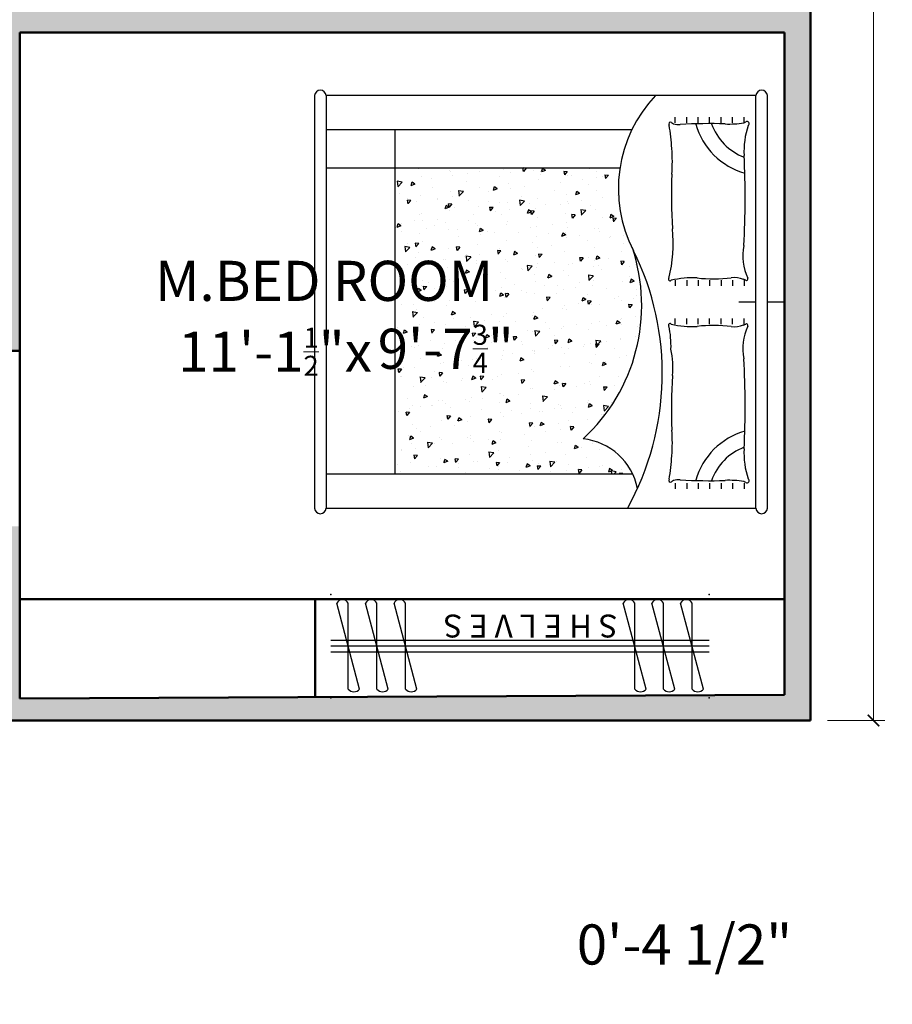
# Model space of a CAD drawing. Units: inches. Extents: x 4508 to 5907, y 877 to 1592.
# Tile 8 of 20: x 5392 to 5544, y 877 to 1049. Entities that reach past the tile are written whole.
import ezdxf

# ---------------------------------------------------------------- set-up
doc = ezdxf.new("R2010")
doc.units = ezdxf.units.IN
doc.layers.get('DEFPOINTS').update_dxf_attribs({"color": 8})
for name, color, linetype, lineweight in [('A-ANNO-DIMS', 2, 'Continuous', 18), ('A-FURN', 24, 'Continuous', 18), ('A-WALL', 7, 'Continuous', 50), ('A-WALL-PATT', 8, 'Continuous', 13)]:
    doc.layers.add(name, color=color, linetype=linetype, lineweight=lineweight)
doc.layers.add('furniture', color=24, linetype='Continuous')
doc.styles.get("Standard").update_dxf_attribs({"font": 'arial.ttf'})
doc.dimstyles.new('details', dxfattribs={"dimtxt": 5, "dimasz": 2, "dimexe": 2, "dimexo": 3, "dimgap": 1, "dimtad": 0, "dimdec": 1, "dimzin": 0, "dimdsep": 46, "dimlunit": 4, "dimtxsty": 'Standard', "dimblk": 'ARCHTICK', "dimcen": 3, "dimclrd": 256, "dimclre": 256, "dimclrt": 256, "dimadec": 0, "dimazin": 0, "dimtfac": 0.5, "dimtdec": 1, "dimtofl": 0, "dimtmove": 0, "dimatfit": 3, "dimldrblk": 'CLOSEDBLANK', "dimfxl": 2, "dimtolj": 1, "dimtzin": 0, "dimlwd": -1, "dimlwe": -1, "dimarcsym": 0})
doc.dimstyles.new('text', dxfattribs={"dimtxt": 7, "dimasz": 0, "dimexe": 3, "dimexo": 3, "dimgap": 0, "dimtad": 1, "dimtih": 1, "dimtoh": 1, "dimzin": 3, "dimdsep": 46, "dimlunit": 4, "dimtxsty": 'Standard', "dimblk": 'CLOSEDBLANK', "dimcen": 3, "dimse1": 1, "dimse2": 1, "dimsd1": 1, "dimsd2": 1, "dimclrd": 256, "dimclre": 256, "dimclrt": 256, "dimadec": 0, "dimazin": 0, "dimtfac": 0.5, "dimtofl": 0, "dimtmove": 0, "dimatfit": 3, "dimfxl": 3, "dimtolj": 1, "dimtzin": 0, "dimlwd": -1, "dimlwe": -1, "dimarcsym": 0})

# ---------------------------------------------------------------- blocks, each defined once
blk = doc.blocks.new('bed')
at = {"layer": 'furniture'}
h = blk.add_hatch(dxfattribs=at)
h.set_pattern_fill('AR-CONC', color=256, angle=-90, style=0)
h.set_pattern_definition([(320, (0, 2.38), (-0.6275, -7.1726), [0.75, -8.25]), (265, (0, 2.38), (7.5219, 1.3875), [0.6, -6.6]), (10.451, (-0.052, 1.782), (6.8944, -5.7851), [0.6374, -7.0114]), (316.184, (2, 2.38), (-1.6552, -10.6724), [1.125, -12.375]), (6.636, (1.862, 1.491), (9.7412, -9.3466), [0.9561, -10.5171]), (261.184, (2, 2.38), (9.7412, -9.3466), [0.9, -9.9]), (291, (1.5, 1.38), (-4.0262, -5.96907), [0.75, -8.25]), (236, (1.5, 1.38), (7.2515, -2.43315), [0.6, -6.6]), (341.451, (1.1645, 0.8826), (3.2253, -8.4022), [0.6374, -7.0114]), (307.5, (0, 2.38), (3.32894, -0.1216), [0, -6.52, 0, -6.7, 0, -6.625]), (277.5, (0, 2.38), (3.94412, -2.6307), [0, -3.82, 0, -6.37, 0, -2.525]), (237.5, (0, 4.61), (-0.22555, -5.33822), [0, -2.5, 0, -7.8, 0, -10.35]), (227.5, (0, 5.61), (1.00105, -5.83186), [0, -3.25, 0, -5.18, 0, -7.35])])
h.paths.add_polyline_path([(30.01, -68), (30.01, -26.5, 0.263043), (23.9, -35.15, 0.293424), (-9.18, -26.47, -0.156683), (-23.39, -28.72), (-23.39, -68)])
for p, q in [((0, -3), (0, 0)), ((36.01, -3), (-36.01, -3)), ((-36.01, -5), (-36.01, -80)), ((36.01, -5), (-36.01, -5)), ((0, -8), (0, -5)), ((36.01, -80), (36.01, -5)), ((-31.24, -7.07), (-32.24, -7.07)), ((-3.81, -7.07), (-2.81, -7.07)), ((3.89, -7.07), (2.89, -7.07)), ((31.63, -7.07), (32.63, -7.07)), ((-31.24, -9.07), (-32.24, -9.07)), ((-3.81, -9.07), (-2.81, -9.07)), ((3.89, -9.07), (2.89, -9.07)), ((31.63, -9.07), (32.63, -9.07)), ((-31.24, -11.07), (-32.24, -11.07)), ((-3.81, -11.07), (-2.81, -11.07)), ((3.89, -11.07), (2.89, -11.07)), ((31.63, -11.07), (32.63, -11.07)), ((-31.24, -13.07), (-32.24, -13.07)), ((-3.81, -13.07), (-2.81, -13.07)), ((3.89, -13.07), (2.89, -13.07)), ((31.63, -13.07), (32.63, -13.07)), ((-31.24, -15.07), (-32.24, -15.07)), ((-3.81, -15.07), (-2.81, -15.07)), ((3.89, -15.07), (2.89, -15.07)), ((31.63, -15.07), (32.63, -15.07)), ((-31.24, -17.07), (-32.24, -17.07)), ((-3.81, -17.07), (-2.81, -17.07)), ((3.89, -17.07), (2.89, -17.07)), ((31.63, -17.07), (32.63, -17.07)), ((-31.24, -19.07), (-32.24, -19.07)), ((-3.81, -19.07), (-2.81, -19.07)), ((3.89, -19.07), (2.89, -19.07)), ((31.63, -19.07), (32.63, -19.07)), ((-36.01, -80), (36.01, -80)), ((-36.01, -82), (36.01, -82))]:
    blk.add_line(p, q, dxfattribs=at)
at = {"layer": 'furniture', "ltscale": 5}
blk.add_line((-30.01, -26.66), (-30.01, -80), dxfattribs=at)
at = {"layer": 'furniture', "ltscale": 7}
blk.add_line((30.01, -80), (30.01, -26.5), dxfattribs=at)
at = {"layer": 'furniture', "ltscale": 0.3}
for p, q in [((-23.39, -80), (-23.39, -28.72)), ((-30.01, -68), (30.01, -68))]:
    blk.add_line(p, q, dxfattribs=at)
at = {"layer": 'furniture'}
for centre, radius, start, end in [((-35.95, -4), 1, 93.3831, 266.6169), ((35.95, -4), 1, 273.3831, 86.6169), ((-31.1, -6.57), 0.382, 35.8976, 208.6272), ((-44.44, -13.85), 14.82, 27.1629, 28.6272), ((-26.35, 6.68), 13.76, 251.1782, 273.3982), ((-8.03, 2.03), 9.29, 258.896, 294.7184), ((-4.03, -6.67), 0.282, 335.7259, 114.303), ((3.22, -9.94), 7.68, 155.7259, 159.0146), ((4.11, -6.67), 0.282, 65.697, 204.2741), ((-3.14, -9.94), 7.68, 20.9854, 24.2741), ((8.12, 2.03), 9.29, 245.2816, 281.104), ((26.43, 6.68), 13.76, 266.6018, 288.8218), ((31.18, -6.57), 0.382, 331.3728, 144.1024), ((44.53, -13.85), 14.82, 151.3728, 152.8371), ((-46.76, -9.65), 15.72, 357.4804, 9.3956), ((-34.45, -3.51), 9.85, 289.8695, 338.9843), ((-34.45, -3.51), 12.47, 286.0319, 344.1205), ((-18.02, -163.6), 156.72, 87.0032, 92.7497), ((0.25, -8.8), 4.49, 159.0146, 186.273), ((-0.17, -8.8), 4.49, 353.727, 20.9854), ((18.1, -163.6), 156.72, 87.2503, 92.9968), ((34.54, -3.51), 12.47, 195.8795, 253.9681), ((34.54, -3.51), 9.85, 201.0157, 250.1305), ((46.84, -9.65), 15.72, 170.6044, 182.5196), ((-32.82, -12.44), 28.78, 354.3784, 6.273), ((32.9, -12.44), 28.78, 173.727, 185.6216), ((-28.62, 31.03), 42.31, 266.4836, 266.6487), ((54.88, -13.16), 85.99, 178.1209, 183.3613), ((-54.8, -13.16), 85.99, 356.6387, 1.8791), ((28.7, 31.03), 42.31, 273.3513, 273.5164), ((12.28, -16.11), 16.48, 177.0317, 192.8678), ((-12.19, -16.11), 16.48, 347.1322, 2.9683), ((-34.13, -18.41), 3.18, 342.7809, 3.755), ((34.21, -18.41), 3.18, 176.245, 197.2191), ((-31.05, -19.91), 0.291, 147.6219, 311.9343), ((-33.2, -18.55), 2.25, 327.6219, 339.2246), ((-24.4, -58.01), 38.42, 93.5164, 99.6766), ((-24.52, -56.06), 36.48, 86.4836, 93.5164), ((-18.49, 70.49), 90.23, 267.5921, 273.6329), ((-10.31, -44.95), 25.52, 75.952, 95.5452), ((-3.95, -19.99), 0.265, 231.9005, 52.8902), ((4.03, -19.99), 0.265, 127.1098, 308.0995), ((7.57, -34.68), 14.87, 87.3976, 103.1191), ((11.44, -34.81), 15.32, 84.694, 102.0355), ((18.57, 70.49), 90.23, 266.3671, 272.4079), ((24.6, -56.06), 36.48, 86.4836, 93.5164), ((24.48, -58.01), 38.42, 80.3234, 86.4836), ((31.13, -19.91), 0.291, 228.0657, 32.3781), ((33.28, -18.55), 2.25, 200.7754, 212.3781), ((12.51, -69.71), 48.38, 60.9345, 116.3227), ((-19.79, -5.47), 23.53, 226.4061, 297.4441), ((0.6, -56.57), 31.65, 42.5874, 108.5034), ((34.61, -36.23), 10.76, 101.1719, 174.259), ((-35.95, -81), 1, 93.3831, 266.6169), ((35.95, -81), 1, 273.3831, 86.6169)]:
    blk.add_arc(centre, radius, start, end, dxfattribs=at)
blk = doc.blocks.new('*D109')
at = {"layer": 'DEFPOINTS', "color": 0, "transparency": 16777216}
for p in [(5460.86, 1046.7), (5455.62, 930.84), (5466.29, 930.84)]:
    blk.add_point(p, dxfattribs=at)
at = {"layer": 'A-ANNO-DIMS', "color": 0, "transparency": 16777216, "insert": (5466.29, 991.53), "char_height": 7, "width": 32.6217, "attachment_point": 5}
blk.add_mtext('\\A1;9\'-7{\\H0.5x;\\S3/4;}"', dxfattribs=at)
blk = doc.blocks.new('_ClosedBlank')
at = {"color": 0, "lineweight": -2}
for p, q in [((-1, 0.167), (0, 0)), ((-1, 0.167), (-1, -0.167)), ((0, 0), (-1, -0.167))]:
    blk.add_line(p, q, dxfattribs=at)
blk = doc.blocks.new('*D110')
at = {"layer": 'DEFPOINTS', "color": 0, "transparency": 16777216}
for p in [(5525.4, 986.86), (5391.95, 982.69), (5525.4, 975.67)]:
    blk.add_point(p, dxfattribs=at)
at = {"layer": 'A-ANNO-DIMS', "color": 0, "transparency": 16777216, "insert": (5436.51, 996.85), "char_height": 7, "attachment_point": 5}
blk.add_mtext('\\A1;        M.BED ROOM\\P11\'-1{\\H0.5x;\\S1/2;}"x', dxfattribs=at)
blk = doc.blocks.new('hangers')
at = {"layer": 'furniture'}
for p, q in [((1, 7.5), (5, -7.5)), ((3, 7.5), (3, -7.5)), ((6, 7.5), (10, -7.5)), ((8, 7.5), (8, -7.5)), ((11, 7.5), (15, -7.5)), ((13, 7.5), (13, -7.5)), ((51, 7.5), (55, -7.5)), ((53, 7.5), (53, -7.5)), ((56, 7.5), (60, -7.5)), ((58, 7.5), (58, -7.5)), ((61, 7.5), (65, -7.5)), ((63, 7.5), (63, -7.5)), ((66, 1), (0, 1)), ((0, 0), (66, 0)), ((0, -1), (66, -1))]:
    blk.add_line(p, q, dxfattribs=at)
for centre, radius, start, end in [((2, 6.62), 1.33, 41.2884, 138.7116), ((7, 6.62), 1.33, 41.2884, 138.7116), ((12, 6.62), 1.33, 41.2884, 138.7116), ((52, 6.62), 1.33, 41.2884, 138.7116), ((57, 6.62), 1.33, 41.2884, 138.7116), ((62, 6.62), 1.33, 41.2884, 138.7116), ((4, -7.08), 1.08, 202.5549, 337.4451), ((9, -7.08), 1.08, 202.5549, 337.4451), ((14, -7.08), 1.08, 202.5549, 337.4451), ((54, -7.08), 1.08, 202.5549, 337.4451), ((59, -7.08), 1.08, 202.5549, 337.4451), ((64, -7.08), 1.08, 202.5549, 337.4451)]:
    blk.add_arc(centre, radius, start, end, dxfattribs=at)
for p in [(0, 9), (66, 9), (0, -9), (66, -9)]:
    blk.add_point(p, dxfattribs=at)
blk.add_text('S H E L V E S', height=4, dxfattribs=at).set_placement((16, -5.52))
blk = doc.blocks.new('_ArchTick')
at = {"color": 0, "linetype": 'ByBlock', "const_width": 0.15}
blk.add_lwpolyline([(-0.5, -0.5), (0.5, 0.5)], dxfattribs=at)
blk = doc.blocks.new('*D113')
at = {"layer": 'A-ANNO-DIMS', "color": 0, "transparency": 16777216}
for p, q in [((5532.9, 1574.7), (5542.92, 1574.7)), ((5540.92, 1574.7), (5540.92, 1255.95)), ((5540.92, 926.7), (5540.92, 1245.46)), ((5532.9, 926.7), (5542.92, 926.7))]:
    blk.add_line(p, q, dxfattribs=at)
at = {"layer": 'DEFPOINTS', "color": 0, "transparency": 16777216}
for p in [(5529.9, 1574.7), (5540.92, 1574.7), (5529.9, 926.7)]:
    blk.add_point(p, dxfattribs=at)
at = {"layer": 'A-ANNO-DIMS', "color": 0, "transparency": 16777216, "xscale": 2, "yscale": 2, "zscale": 2}
for p, rotation in [((5540.92, 1574.7), 90), ((5540.92, 926.7), 270)]:
    blk.add_blockref('_ArchTick', p, dxfattribs=dict(at, rotation=rotation))
at = {"layer": 'A-ANNO-DIMS', "color": 0, "transparency": 16777216, "insert": (5540.92, 1250.7), "char_height": 5, "attachment_point": 5, "rotation": 90}
blk.add_mtext("\\A1;54'", dxfattribs=at)
blk = doc.blocks.new('*D189')
at = {"layer": 'DEFPOINTS', "color": 0, "transparency": 16777216}
for p in [(5525.4, 931.18), (5529.9, 926.7), (5529.9, 883.98)]:
    blk.add_point(p, dxfattribs=at)
at = {"layer": 'A-ANNO-DIMS', "transparency": 16777216, "insert": (5507.94, 887.6), "char_height": 7, "attachment_point": 5}
blk.add_mtext('\\A1;0\'-4 1/2"', dxfattribs=at)

msp = doc.modelspace()

# ---------------------------------------------------------------- hatches: boundary and pattern name
at = {"layer": 'A-WALL-PATT'}
h = msp.add_hatch(color=256, dxfattribs=at)
h.dxf.hatch_style = 1
h.paths.add_polyline_path([(5529.903, 1303.204), (5388.02, 1303.204), (5388.02, 1294.204), (5391.903, 1294.204), (5391.903, 1205.704), (5396.403, 1205.704), (5396.403, 1294.204), (5489.403, 1294.204), (5489.403, 1256.139), (5493.903, 1256.139), (5493.903, 1294.204), (5529.903, 1294.204)], flags=17)
h.paths.add_polyline_path([(5346.02, 1303.204), (5322.903, 1303.204), (5322.903, 1321.388), (5313.903, 1321.388), (5313.903, 1303.204), (5259.903, 1303.204), (5259.903, 1381.204), (5313.903, 1381.204), (5313.903, 1359.674), (5322.903, 1359.674), (5322.903, 1381.204), (5338.979, 1381.204), (5338.979, 1390.204), (5331.903, 1390.204), (5331.903, 1442.704), (5255.403, 1442.704), (5255.403, 1570.204), (5387.403, 1570.204), (5387.403, 1541.271), (5391.903, 1541.271), (5391.903, 1570.204), (5483.403, 1570.204), (5483.403, 1498.204), (5391.903, 1498.204), (5391.903, 1509.559), (5387.403, 1509.559), (5387.403, 1390.204), (5380.979, 1390.204), (5380.979, 1381.204), (5387.403, 1381.204), (5529.903, 1381.204), (5529.903, 1498.204), (5487.903, 1498.204), (5487.903, 1570.204), (5529.903, 1570.204), (5529.903, 1574.704), (5250.903, 1574.704), (5250.903, 991.204), (5310.903, 991.204), (5310.903, 926.704), (5529.903, 926.704), (5529.903, 1210.204), (5525.403, 1210.204), (5525.403, 1103.704), (5499.903, 1103.704), (5499.903, 1210.204), (5493.903, 1210.204), (5493.903, 1256.139), (5489.403, 1256.139), (5489.403, 1210.204), (5461.584, 1210.204), (5461.584, 1205.704), (5495.403, 1205.704), (5495.403, 1103.704), (5436.903, 1103.704), (5436.903, 1051.204), (5391.954, 1051.204), (5391.954, 1103.03), (5391.954, 1107.53), (5255.403, 1108.204), (5255.403, 1294.204), (5346.02, 1294.204)])
h.paths.add_polyline_path([(5255.403, 1390.204), (5255.403, 1398.204), (5255.403, 1438.204), (5257.903, 1438.204), (5258.903, 1438.204), (5327.403, 1438.204), (5327.403, 1390.204), (5325.903, 1390.204)], flags=16)
h.paths.add_polyline_path([(5288.757, 1390.704), (5288.757, 1390.204), (5292.173, 1390.204), (5292.173, 1390.704)], flags=0)
h.paths.add_polyline_path([(5289.965, 1391.606), (5289.965, 1396.645), (5289.903, 1396.645), (5289.903, 1397.319), (5288.849, 1398.862), (5288.849, 1398.8), (5288.983, 1398.748), (5288.983, 1399.204), (5289.091, 1399.204), (5292.081, 1399.204), (5292.081, 1398.665), (5291.946, 1398.665), (5291.027, 1397.319), (5291.027, 1396.645), (5290.965, 1396.645), (5290.965, 1391.606)], flags=0)
h.paths.add_polyline_path([(5288.849, 1399.069, 2.6374395), (5289.056, 1398.835), (5289.117, 1399.087, 0.9346155)], flags=0)
h.paths.add_polyline_path([(5290.061, 1398.665), (5290.061, 1399.204), (5290.038, 1398.975)], flags=0)
h.paths.add_polyline_path([(5291.946, 1398.934, -1), (5291.946, 1398.665)], flags=0)
h.paths.add_polyline_path([(5289.414, 1398.967), (5289.414, 1399.204), (5289.63, 1399.204), (5289.63, 1398.363), (5290.051, 1397.184), (5290.76, 1397.184), (5290.869, 1398.665), (5290.869, 1399.204), (5290.815, 1398.665), (5290.815, 1399.204), (5291.462, 1399.204), (5291.462, 1398.816), (5290.879, 1397.184), (5290.051, 1397.184)], flags=0)
h.paths.add_polyline_path([(5273.903, 1392.056), (5269.591, 1392.056, 0.0901028), (5265.544, 1392.842), (5265.511, 1392.034, -0.3516542), (5265.903, 1391.546, -1), (5264.903, 1391.546, -0.3042165), (5265.213, 1392.008), (5265.167, 1392.84, 0.0880132), (5261.215, 1392.056), (5256.903, 1392.056), (5256.903, 1398.704, -0.4142136), (5259.403, 1401.204), (5271.403, 1401.204, -0.4142136), (5273.903, 1398.704)], flags=0)
h.paths.add_polyline_path([(5263.726, 1395.073, -1), (5267.08, 1395.073, -1)], flags=0)
h.paths.add_polyline_path([(5264.434, 1395.073, -0.695521), (5265.153, 1395.073, -1.1408699), (5265.403, 1395.585, -0.7522125), (5265.403, 1396.25, 0.3674806)], flags=0)
h.paths.add_polyline_path([(5265.153, 1394.399, -1), (5265.653, 1394.399, -1)], flags=0)
h.paths.add_polyline_path([(5265.905, 1395.077, -1), (5266.405, 1395.077, -1)], flags=0)
h.paths.add_polyline_path([(5307.994, 1403.113, -1), (5307.994, 1417.295), (5318.794, 1417.295, -0.4142136), (5319.794, 1416.295), (5320.794, 1416.295, -0.4142136), (5321.794, 1417.295), (5324.903, 1417.295, -0.4142136), (5325.903, 1416.295), (5325.903, 1404.113, -0.4142136), (5324.903, 1403.113), (5321.794, 1403.113, -0.4142136), (5320.794, 1404.113), (5319.794, 1404.113, -0.4142136), (5318.794, 1403.113)], flags=0)
h.paths.add_polyline_path([(5307.836, 1405.113, -1), (5307.836, 1415.295), (5315.591, 1415.295, -0.4142136), (5317.532, 1413.353), (5317.532, 1407.054, -0.4142136), (5315.591, 1405.113)], flags=0)
h.paths.add_polyline_path([(5312.032, 1408.204, -1), (5312.032, 1412.204), (5315.032, 1412.204, -0.4142136), (5316.032, 1411.204), (5316.032, 1409.204, -0.4142136), (5315.032, 1408.204)], flags=0)
h.paths.add_polyline_path([(5391.903, 1385.704), (5391.903, 1493.704), (5525.403, 1493.704), (5525.403, 1385.704)], flags=16)
h.paths.add_polyline_path([(5422.641, 1390.704), (5422.641, 1465.704, -0.9426302), (5422.641, 1467.704), (5494.547, 1467.704, -1), (5494.665, 1465.704), (5494.665, 1390.704, -0.9426302), (5494.665, 1388.704), (5422.759, 1388.704, -1)], flags=0)
h.paths.add_polyline_path([(5427.52, 1395.749, -0.0238564), (5427.614, 1403.949, 0.0884332), (5427.476, 1405.056, 0.0506693), (5427.273, 1405.463, -0.8716827), (5427.713, 1405.835, 0.0268855), (5431.815, 1405.361, 0.0306964), (5436.289, 1405.361, -0.0263641), (5445.798, 1405.259, 0.075811), (5450.408, 1405.53, 0.0687062), (5454.457, 1405.903, -1.0086747), (5454.781, 1405.482, 0.0692081), (5454.389, 1400.959, -0.0519468), (5454.356, 1394.996, 0.1195012), (5454.627, 1392.895, 0.0143508), (5454.796, 1392.489, -0.6962059), (5454.42, 1392.118, 0.1574808), (5448.747, 1392.794, -0.025536), (5432.749, 1392.774, 0.0920085), (5427.781, 1392.048, -0.9384848), (5427.137, 1392.455, 0.0063894), (5427.314, 1392.79, 0.0472995)], flags=0)
h.paths.add_polyline_path([(5426.125, 1411.372, 0.0617649), (5428.641, 1412.201), (5428.641, 1465.704), (5488.665, 1465.704), (5488.665, 1412.363, 0.2363822), (5467.6, 1412.052, -0.2252042)], flags=0)
h.paths.add_polyline_path([(5391.903, 1490.204), (5391.903, 1491.204), (5422.903, 1491.204), (5422.903, 1490.204)], flags=0)
h.paths.add_polyline_path([(5462.545, 1392.771, 0.1270318), (5462.866, 1394.996, -0.0519468), (5462.832, 1400.959, 0.0692081), (5462.441, 1405.482, -1.0086747), (5462.765, 1405.903, 0.0857004), (5471.424, 1405.259, -0.0263641), (5480.932, 1405.361, 0.0306964), (5485.407, 1405.361, 0.0268855), (5489.509, 1405.835, -0.8716827), (5489.949, 1405.463, 0.0506693), (5489.746, 1405.056, 0.0884332), (5489.608, 1403.949, -0.0238564), (5489.702, 1395.749, 0.0472995), (5489.908, 1392.79, 0.0063894), (5490.085, 1392.455, -0.9384848), (5489.441, 1392.048, 0.0920085), (5484.473, 1392.774, -0.025536), (5468.475, 1392.794, 0.1574808), (5462.802, 1392.118, -0.6962059), (5462.426, 1392.489, 0.0100173), (5462.546, 1392.771)], flags=0)
h.paths.add_polyline_path([(5387.454, 1103.03), (5387.454, 1100.53), (5387.454, 1099.53), (5387.454, 995.03), (5387.454, 991.204), (5391.954, 991.204), (5391.954, 1046.704), (5525.403, 1046.704), (5525.403, 931.182), (5391.954, 930.53), (5391.954, 960.53), (5387.454, 960.53), (5387.454, 930.53), (5315.403, 930.53), (5315.403, 991.204), (5323.403, 991.204), (5387.454, 991.204), (5387.454, 995.03), (5255.403, 995.704), (5255.403, 1103.704)], flags=16)
h.paths.add_polyline_path([(5379.264, 1062.889), (5379.264, 1060.156), (5385.764, 1061.889, -0.4526903), (5385.764, 1059.889), (5379.264, 1059.889), (5379.264, 1055.156), (5385.764, 1056.889, -0.4526903), (5385.764, 1054.889), (5379.264, 1054.889), (5379.264, 1050.156), (5385.764, 1051.889, -0.4526903), (5385.764, 1049.889), (5379.264, 1049.889), (5379.264, 1010.156), (5385.764, 1011.889, -0.4526903), (5385.764, 1009.889), (5379.264, 1009.889), (5379.264, 1005.156), (5385.764, 1006.889, -0.4526903), (5385.764, 1004.889), (5379.264, 1004.889), (5379.264, 1000.156), (5385.764, 1001.889, -0.4526903), (5385.764, 999.889), (5378.264, 999.889), (5370.764, 997.889, -0.6674863), (5370.764, 999.889), (5377.264, 999.889), (5377.264, 1004.623), (5370.764, 1002.889, -0.6674863), (5370.764, 1004.889), (5377.264, 1004.889), (5377.264, 1009.623), (5370.764, 1007.889, -0.6674863), (5370.764, 1009.889), (5377.264, 1009.889), (5377.264, 1049.623), (5370.764, 1047.889, -0.6674863), (5370.764, 1049.889), (5377.264, 1049.889), (5377.264, 1054.623), (5370.764, 1052.889, -0.6674863), (5370.764, 1054.889), (5377.264, 1054.889), (5377.264, 1059.623), (5370.764, 1057.889, -0.6674863), (5370.764, 1059.889), (5377.264, 1059.889), (5377.264, 1062.889)], flags=0)
h.paths.add_polyline_path([(5287.641, 1000.704), (5359.665, 1000.704), (5359.665, 1018.212, 0.3202856), (5332.6, 1022.052, -0.246494), (5287.641, 1023.128)], flags=0)
h.paths.add_polyline_path([(5359.547, 1077.704, -1), (5359.665, 1075.704), (5353.665, 1075.704), (5353.665, 1063.704), (5293.641, 1063.704), (5293.641, 1075.704), (5287.759, 1075.704, -1), (5287.641, 1077.704)], flags=0)
h.paths.add_polyline_path([(5441.403, 1099.204), (5525.403, 1099.204), (5525.403, 1051.204), (5441.403, 1051.204), (5441.403, 1059.204)], flags=16)
h.paths.add_polyline_path([(5441.403, 1096.704), (5466.403, 1096.704), (5466.403, 1095.704), (5441.403, 1095.704)], flags=0)
h.paths.add_polyline_path([(5445.403, 1062.204), (5457.403, 1062.204, -0.4142136), (5459.903, 1059.704), (5459.903, 1053.056), (5455.591, 1053.056, 0.0901028), (5451.544, 1053.842), (5451.511, 1053.034, -0.3516542), (5451.903, 1052.546, -1), (5450.903, 1052.546, -0.3042165), (5451.213, 1053.008), (5451.167, 1053.84, 0.0880132), (5447.215, 1053.056), (5442.903, 1053.056), (5442.903, 1059.704, -0.4142136)], flags=0)
h.paths.add_polyline_path([(5453.08, 1056.073, -1), (5449.726, 1056.073, -1)], flags=0)
h.paths.add_polyline_path([(5292.713, 1015.835, 0.0268855), (5296.815, 1015.361, 0.0306964), (5301.289, 1015.361, -0.0263641), (5310.798, 1015.259, 0.075811), (5315.408, 1015.53, 0.0687062), (5319.457, 1015.903, -1.0086747), (5319.781, 1015.482, 0.0692081), (5319.389, 1010.959, -0.0519468), (5319.356, 1004.996, 0.1195012), (5319.627, 1002.895, 0.0143508), (5319.796, 1002.489, -0.6962059), (5319.42, 1002.118, 0.1574808), (5313.747, 1002.794, -0.025536), (5297.749, 1002.774, 0.0920085), (5292.781, 1002.048, -0.9384848), (5292.137, 1002.455, 0.0063894), (5292.314, 1002.79, 0.0472995), (5292.52, 1005.749, -0.0238564), (5292.614, 1013.949, 0.0884332), (5292.476, 1015.056, 0.0506693), (5292.273, 1015.463, -0.8716827)], flags=0)
h.paths.add_polyline_path([(5450.434, 1056.073, -0.695521), (5451.153, 1056.073, -1.1408699), (5451.403, 1056.585, -0.7522125), (5451.403, 1057.25, 0.3674806)], flags=0)
h.paths.add_polyline_path([(5327.765, 1015.903, 0.0857004), (5336.424, 1015.259, -0.0263641), (5345.932, 1015.361, 0.0306964), (5350.407, 1015.361, 0.0268855), (5354.509, 1015.835, -0.8716827), (5354.949, 1015.463, 0.0506693), (5354.746, 1015.056, 0.0884332), (5354.608, 1013.949, -0.0238564), (5354.702, 1005.749, 0.0472995), (5354.908, 1002.79, 0.0063894), (5355.085, 1002.455, -0.9384848), (5354.441, 1002.048, 0.0920085), (5349.473, 1002.774, -0.025536), (5333.475, 1002.794, 0.1574808), (5327.802, 1002.118, -0.6962059), (5327.426, 1002.489, 0.0100173), (5327.546, 1002.771), (5327.545, 1002.771, 0.1270318), (5327.866, 1004.996, -0.0519468), (5327.832, 1010.959, 0.0692081), (5327.441, 1015.482, -1.0086747)], flags=0)
h.paths.add_polyline_path([(5452.405, 1056.077, -1), (5451.905, 1056.077, -1)], flags=0)
h.paths.add_polyline_path([(5451.653, 1055.399, -1), (5451.153, 1055.399, -1)], flags=0)
h.paths.add_polyline_path([(5472.958, 1051.704), (5472.958, 1051.204), (5476.374, 1051.204), (5476.374, 1051.704)], flags=0)
h.paths.add_polyline_path([(5476.282, 1060.204), (5476.282, 1059.665), (5476.147, 1059.665), (5475.228, 1058.319), (5475.228, 1057.645), (5475.166, 1052.606), (5474.166, 1052.606), (5474.166, 1057.645), (5474.104, 1057.645), (5474.104, 1058.319), (5473.05, 1059.862), (5473.05, 1059.8), (5473.184, 1059.748), (5473.184, 1060.204), (5473.292, 1060.204)], flags=0)
h.paths.add_polyline_path([(5473.05, 1060.069, 2.6374395), (5473.257, 1059.835), (5473.318, 1060.087, 0.9346155)], flags=0)
h.paths.add_polyline_path([(5473.831, 1060.204), (5473.831, 1059.363), (5474.252, 1058.184), (5474.371, 1058.184), (5474.262, 1059.665), (5474.262, 1060.204)], flags=0)
h.paths.add_polyline_path([(5475.501, 1060.204), (5475.501, 1059.363), (5475.555, 1059.514), (5475.555, 1060.204)], flags=0)
h.paths.add_polyline_path([(5474.855, 1060.204), (5474.908, 1060.127), (5474.908, 1060.204), (5474.855, 1059.665)], flags=0)
h.paths.add_polyline_path([(5476.147, 1059.934, -1), (5476.147, 1059.665)], flags=0)
h.paths.add_polyline_path([(5474.693, 1060.204), (5475.178, 1059.511), (5475.178, 1060.204), (5475.285, 1059.934), (5475.285, 1060.204), (5475.178, 1059.665), (5475.178, 1060.204), (5475.07, 1059.665), (5475.07, 1060.204), (5474.962, 1059.665), (5474.962, 1060.204), (5474.693, 1059.306)], flags=0)
h.paths.add_polyline_path([(5474.747, 1060.204), (5474.37, 1059.45), (5474.37, 1060.204), (5474.424, 1060.096), (5474.424, 1060.204), (5474.747, 1059.665)], flags=0)
h.paths.add_polyline_path([(5476.04, 1059.665), (5476.04, 1060.204), (5476.094, 1059.665), (5476.094, 1060.204)], flags=0)
h.paths.add_polyline_path([(5505.994, 1082.295), (5516.794, 1082.295, -0.4142136), (5517.794, 1081.295), (5518.794, 1081.295, -0.4142136), (5519.794, 1082.295), (5522.903, 1082.295, -0.4142136), (5523.903, 1081.295), (5523.903, 1069.113, -0.4142136), (5522.903, 1068.113), (5519.794, 1068.113, -0.4142136), (5518.794, 1069.113), (5517.794, 1069.113, -0.4142136), (5516.794, 1068.113), (5505.994, 1068.113, -1)], flags=0)
h.paths.add_polyline_path([(5505.836, 1080.295), (5513.591, 1080.295, -0.4142136), (5515.532, 1078.353), (5515.532, 1072.054, -0.4142136), (5513.591, 1070.113), (5505.836, 1070.113, -1)], flags=0)
h.paths.add_polyline_path([(5520.403, 963.695), (5520.403, 1035.72), (5502.895, 1035.72, 0.3202856), (5499.055, 1008.654, -0.246494), (5497.978, 963.695)], flags=0)
h.paths.add_polyline_path([(5445.403, 1035.72), (5445.403, 1029.72), (5457.403, 1029.72), (5457.403, 969.695), (5445.403, 969.695), (5445.403, 963.814, -1), (5443.403, 963.695), (5443.403, 1035.602, -1)], flags=0)
h.paths.add_polyline_path([(5510.032, 1077.204), (5513.032, 1077.204, -0.4142136), (5514.032, 1076.204), (5514.032, 1074.204, -0.4142136), (5513.032, 1073.204), (5510.032, 1073.204, -1)], flags=0)
h.paths.add_polyline_path([(5317.255, 989.704), (5323.903, 989.704, -0.4142136), (5326.403, 987.204), (5326.403, 975.204, -0.4142136), (5323.903, 972.704), (5317.255, 972.704), (5317.255, 977.016, 0.0901028), (5318.041, 981.063), (5317.233, 981.096, -0.8964437), (5316.245, 981.204, -0.8220123), (5317.207, 981.394), (5318.04, 981.44, 0.0880132), (5317.255, 985.392)], flags=0)
h.paths.add_polyline_path([(5321.949, 981.204, -1), (5318.594, 981.204, -1)], flags=0)
h.paths.add_polyline_path([(5362.454, 988.03), (5387.454, 988.03), (5387.454, 990.53), (5391.954, 990.53), (5391.704, 988.289, -0.4090807), (5391.204, 987.78), (5391.204, 987.53), (5388.954, 987.53), (5388.954, 988.03), (5387.454, 988.03), (5387.454, 987.03), (5362.474, 987.03, 0.4025427), (5387.454, 963.03), (5388.954, 963.03), (5388.954, 963.53), (5391.195, 963.28, -0.4142136), (5391.704, 962.771), (5391.954, 960.53), (5391.954, 962.78), (5391.704, 962.78, 0.4090807), (5391.195, 963.28), (5388.954, 963.53), (5388.954, 963.03), (5387.454, 963.03, -0.4025427), (5362.474, 987.03), (5362.454, 987.03)], flags=0)
h.paths.add_polyline_path([(5321.285, 981.204, -0.6555366), (5320.522, 981.204, -1.1195284), (5320.275, 980.701, -1.3500746), (5320.279, 980.026, 0.3749463)], flags=0)
h.paths.add_polyline_path([(5320.022, 981.923, -1), (5320.522, 981.923, -1)], flags=0)
h.paths.add_polyline_path([(5319.348, 981.204, -1), (5319.848, 981.204, -1)], flags=0)
h.paths.add_polyline_path([(5507.157, 1030.662, -0.0238564), (5515.358, 1030.756, 0.0472995), (5518.317, 1030.962, 0.0063894), (5518.652, 1031.139, -0.9384848), (5519.059, 1030.495, 0.0920085), (5518.333, 1025.527, -0.025536), (5518.313, 1009.53, 0.1574808), (5518.989, 1003.857, -0.6962059), (5518.618, 1003.48, 0.0100173), (5518.335, 1003.601), (5518.335, 1003.6, 0.1270318), (5516.111, 1003.921, -0.0519468), (5510.148, 1003.887, 0.0692081), (5505.624, 1003.495, -1.0086747), (5505.204, 1003.819, 0.0857004), (5505.848, 1012.479, -0.0263641), (5505.746, 1021.987, 0.0306964), (5505.746, 1026.462, 0.0268855), (5505.272, 1030.563, -0.8716827), (5505.644, 1031.004, 0.0506693), (5506.051, 1030.801, 0.0884332)], flags=0)
h.paths.add_polyline_path([(5368.045, 945.621), (5378.845, 945.621, -0.4142136), (5379.845, 944.621), (5380.845, 944.621, -0.4142136), (5381.845, 945.621), (5384.954, 945.621, -0.4142136), (5385.954, 944.621), (5385.954, 932.439, -0.4142136), (5384.954, 931.439), (5381.845, 931.439, -0.4142136), (5380.845, 932.439), (5379.845, 932.439, -0.4142136), (5378.845, 931.439), (5368.045, 931.439, -1)], flags=0)
h.paths.add_polyline_path([(5327.31, 931.03), (5327.31, 930.53), (5330.726, 930.53), (5330.726, 931.03)], flags=0)
h.paths.add_polyline_path([(5330.634, 939.53), (5330.634, 938.991), (5330.499, 938.991), (5329.579, 937.645), (5329.579, 936.971), (5329.518, 936.971), (5329.518, 931.933), (5328.518, 931.933), (5328.518, 936.971), (5328.456, 936.971), (5328.456, 937.645), (5327.402, 939.189), (5327.402, 939.126), (5327.536, 939.074), (5327.536, 939.53), (5327.644, 939.53)], flags=0)
h.paths.add_polyline_path([(5327.402, 939.395, 2.6374395), (5327.609, 939.161), (5327.67, 939.414, 0.9346155)], flags=0)
h.paths.add_polyline_path([(5328.021, 939.142), (5328.021, 939.53), (5327.967, 939.53), (5327.967, 939.293)], flags=0)
h.paths.add_polyline_path([(5328.614, 939.53), (5328.614, 938.991), (5328.723, 937.51), (5329.313, 937.51), (5329.422, 938.991), (5329.422, 939.53), (5329.368, 938.991), (5329.368, 939.53)], flags=0)
h.paths.add_polyline_path([(5329.853, 939.53), (5329.853, 938.689), (5329.907, 938.84), (5329.907, 939.53)], flags=0)
h.paths.add_polyline_path([(5330.499, 939.261, -1), (5330.499, 938.991)], flags=0)
h.paths.add_polyline_path([(5367.887, 943.621), (5375.641, 943.621, -0.4142136), (5377.583, 941.68), (5377.583, 935.38, -0.4142136), (5375.641, 933.439), (5367.887, 933.439, -1)], flags=0)
h.paths.add_polyline_path([(5509.267, 947.14), (5509.267, 939.64), (5511.267, 932.14, -0.4526903), (5509.267, 932.14), (5509.267, 938.64), (5504.534, 938.64), (5506.267, 932.14, -0.4526903), (5504.267, 932.14), (5504.267, 938.64), (5499.534, 938.64), (5501.267, 932.14, -0.4526903), (5499.267, 932.14), (5499.267, 938.64), (5459.534, 938.64), (5461.267, 932.14, -0.4526903), (5459.267, 932.14), (5459.267, 938.64), (5454.534, 938.64), (5456.267, 932.14, -0.4526903), (5454.267, 932.14), (5454.267, 938.64), (5449.534, 938.64), (5451.267, 932.14, -0.4526903), (5449.267, 932.14), (5449.267, 939.64), (5447.267, 947.14, -0.3030853), (5448.267, 947.808), (5508.266, 947.808, -0.3032033)], flags=0)
h.paths.add_polyline_path([(5510.148, 995.444, -0.0519468), (5516.111, 995.41, 0.1195012), (5518.212, 995.681, 0.0143508), (5518.618, 995.851, -0.6962059), (5518.989, 995.474, 0.1574808), (5518.313, 989.801, -0.025536), (5518.333, 973.804, 0.0920085), (5519.059, 968.836, -0.9384848), (5518.652, 968.192, 0.0063894), (5518.317, 968.369, 0.0472995), (5515.358, 968.575, -0.0238564), (5507.157, 968.669, 0.0884332), (5506.051, 968.531, 0.0506693), (5505.644, 968.327, -0.8716827), (5505.272, 968.768, 0.0268855), (5505.746, 972.869, 0.0306964), (5505.746, 977.344, -0.0263641), (5505.848, 986.852, 0.075811), (5505.576, 991.462, 0.0687062), (5505.204, 995.512, -1.0086747), (5505.624, 995.836, 0.0692081)], flags=0)
h.paths.add_polyline_path([(5372.083, 940.53), (5375.083, 940.53, -0.4142136), (5376.083, 939.53), (5376.083, 937.53, -0.4142136), (5375.083, 936.53), (5372.083, 936.53, -1)], flags=0)
h.paths.add_polyline_path([(5409.258, 1465.643), (5487.738, 1465.643), (5487.738, 1492.394), (5409.258, 1492.394)], flags=8)
h.paths.add_polyline_path([(5463.574, 1465.103), (5486.546, 1465.103), (5486.546, 1479.528), (5463.574, 1479.528)], flags=8)
h.paths.add_polyline_path([(5248.665, 1406.171), (5299.981, 1406.171), (5299.981, 1432.34), (5248.665, 1432.34)], flags=9)
h.paths.add_polyline_path([(5287.471, 1405.121), (5310.443, 1405.121), (5310.443, 1419.546), (5287.471, 1419.546)], flags=8)
h.paths.add_polyline_path([(5371.637, 1047.927), (5371.637, 1010.764), (5377.841, 1010.764), (5377.841, 1047.927)], flags=8)
h.paths.add_polyline_path([(5324.882, 1074.869), (5347.854, 1074.869), (5347.854, 1089.294), (5324.882, 1089.294)], flags=8)
h.paths.add_polyline_path([(5262.863, 1074.665), (5351.123, 1074.665), (5351.123, 1100.833), (5262.863, 1100.833)], flags=8)
h.paths.add_polyline_path([(5307.238, 938.814), (5363.988, 938.814), (5363.988, 964.982), (5307.238, 964.982)], flags=24)
h.paths.add_polyline_path([(5348.837, 937.997), (5371.809, 937.997), (5371.809, 952.422), (5348.837, 952.422)], flags=8)
h.paths.add_polyline_path([(5432.497, 1066.695), (5489.247, 1066.695), (5489.247, 1092.863), (5432.497, 1092.863)], flags=24)
h.paths.add_polyline_path([(5473.52, 1065.943), (5496.492, 1065.943), (5496.492, 1080.368), (5473.52, 1080.368)], flags=8)
h.paths.add_polyline_path([(5451.783, 984.266), (5480.194, 984.266), (5480.194, 998.691), (5451.783, 998.691)], flags=8)
h.paths.add_polyline_path([(5392.211, 983.632), (5481.554, 983.632), (5481.554, 1010.383), (5392.211, 1010.383)], flags=8)
h.paths.add_polyline_path([(5497.304, 946.267), (5460.142, 946.267), (5460.142, 940.062), (5497.304, 940.062)], flags=8)

# ---------------------------------------------------------------- linework, layer by layer
at = {"layer": 'A-WALL'}
for p, q in [((5529.903, 1574.704), (5529.903, 926.704)), ((5391.954, 1046.704), (5525.403, 1046.704)), ((5391.954, 1046.704), (5391.954, 930.53)), ((5525.403, 1046.704), (5525.403, 931.182)), ((5391.954, 947.841), (5525.403, 947.841)), ((5443.509, 947.783), (5443.509, 930.675)), ((5525.403, 931.182), (5391.954, 930.53)), ((5529.903, 926.704), (5250.903, 926.704))]:
    msp.add_line(p, q, dxfattribs=at)
msp.add_lwpolyline([(5387.454, 930.53), (5315.403, 930.53), (5315.403, 991.204), (5391.954, 991.204), (5391.954, 930.53)], dxfattribs=at)

# ---------------------------------------------------------------- block references
at = {"layer": 'A-FURN'}
for name, p, rotation in [('bed', (5525.403, 999.708), 270), ('hangers', (5512.267, 939.64), 180)]:
    msp.add_blockref(name, p, dxfattribs=dict(at, rotation=rotation))

# ---------------------------------------------------------------- dimensions: what is measured, and where the dimension line sits
at = {"layer": 'A-ANNO-DIMS'}
dim = msp.add_linear_dim(base=(5540.921, 1574.704), p1=(5529.903, 926.704), p2=(5529.903, 1574.704), angle=90, dimstyle='details', override={"dimclrd": 0, "dimclre": 0, "dimclrt": 0}, dxfattribs=at)
dim.commit()
dim.dimension.update_dxf_attribs({"geometry": '*D113', "text_midpoint": (5540.921, 1250.704)})
dim = msp.add_linear_dim(base=(5466.292, 930.841), p1=(5460.86, 1046.704), p2=(5455.615, 930.841), angle=90, dimstyle='text', override={"dimclrd": 0, "dimclre": 0, "dimclrt": 0}, dxfattribs=at)
dim.commit()
dim.dimension.update_dxf_attribs({"geometry": '*D109', "text_midpoint": (5466.292, 991.529), "dimtype": 160})
dim = msp.add_linear_dim(base=(5525.403, 986.856), p1=(5391.954, 982.69), p2=(5525.403, 975.672), text='        M.BED ROOM\\P<>x', dimstyle='text', override={"dimclrd": 0, "dimclre": 0, "dimclrt": 0}, dxfattribs=at)
dim.commit()
dim.dimension.update_dxf_attribs({"geometry": '*D110', "text_midpoint": (5436.512, 986.856), "dimtype": 160})
dim = msp.add_linear_dim(base=(5529.903, 883.98), p1=(5525.403, 931.182), p2=(5529.903, 926.704), dimstyle='text', override={"dimdec": 1, "dimlfac": 1, "dimrnd": 0, "dimzin": 1, "dimdsep": 46, "dimlunit": 4, "dimfrac": 2}, dxfattribs=at)
dim.commit()
dim.dimension.update_dxf_attribs({"geometry": '*D189', "text_midpoint": (5507.944, 887.599)})

doc.saveas('drawing.dxf')
